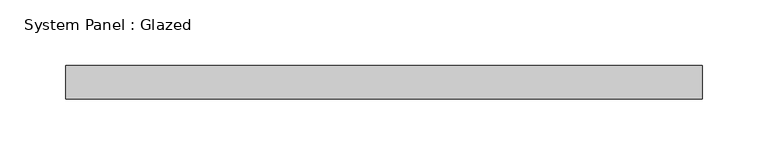
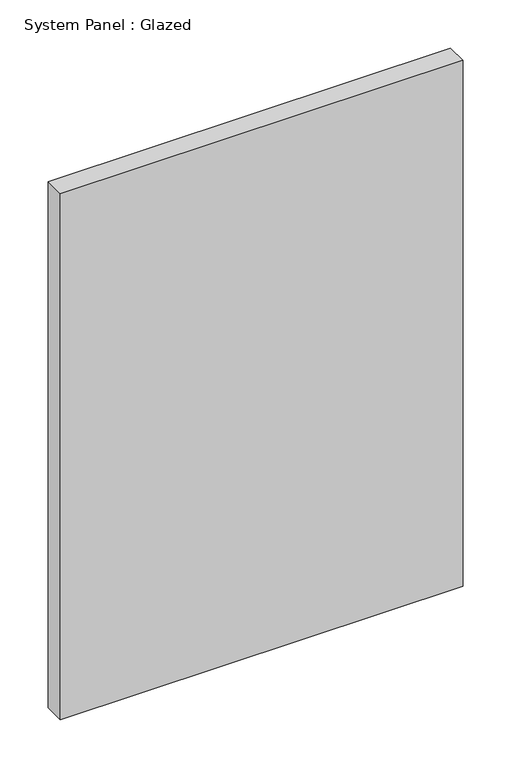
"""IFC4 building model written with IfcOpenShell, lengths in millimetres: plate geometry, System Panel : Glazed."""

from ifc_helpers import new_model, si_unit, origin, origin_with_axes, place, context, project, spatial, polyline, outline, extrude, source, transform, mapped, element, save


def system_panel_glazed_afbb4b88(model_context):
    return source(origin(), model_context, "Body", "SweptSolid", [
        extrude(outline(polyline([(241.3, 19.05), (-241.3, 19.05), (-241.3, 44.45), (241.3, 44.45), (241.3, 19.05)])), origin_with_axes(), (0.0, 0.0, 1.0), 666.75),
    ])


if __name__ == "__main__":
    model = new_model("IFC4")
    model_context = context("Model", 3, world=origin())
    ifc_project = project(units=[si_unit("LENGTHUNIT", "METRE", prefix="MILLI")], contexts=[model_context])
    site = spatial("IfcSite", under=ifc_project)
    building = spatial("IfcBuilding", under=site)
    placement = place(None, origin())
    system_panel_glazed_shape = system_panel_glazed_afbb4b88(model_context)
    element("IfcPlate", 1, ObjectType="System Panel : Glazed", at=placement, inside=building, context=model_context, shape_type="MappedRepresentation", body=[
        mapped(system_panel_glazed_shape, transform((0.0, 0.0, 0.0), x_axis=(1.0, 0.0, 0.0), y_axis=(0.0, 1.0, 0.0), z_axis=(0.0, 0.0, 1.0))),
    ])
    save(model, "model.ifc")

# Revit data of these elements
# Type "System Panel : Glazed"
#   Construction Type Id = "GSP4R"
#   Analytic Construction = "1/8 in Pilkington single glazing"
#   Visual Light Transmittance = 0.9
#   Solar Heat Gain Coefficient = 0.86
#   Heat Transfer Coefficient (U) = 1.18115 BTU/(h·ft²·°F)
#   Define Thermal Properties by = 1
# Element 1 (IfcPlate, "System Panel : Glazed")
#   Materials on its faces: "Glass"
# Materials
#   "Glass": class "Glass", colour RGB 0 128 192, transparency 0.75, Description = "Soda Lime Glass", Cost = 0
